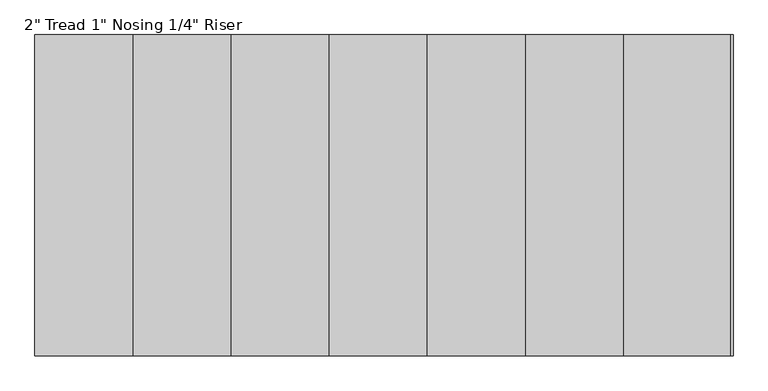
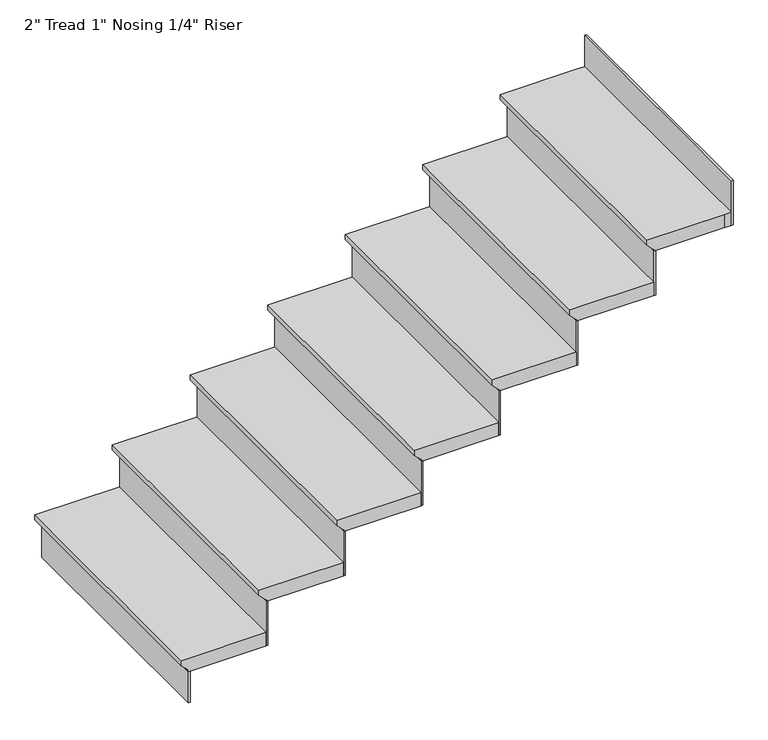
"""IFC4 building model written with IfcOpenShell, lengths in millimetres: stair flight geometry."""

from ifc_helpers import new_model, si_unit, origin, place, context, project, spatial, faceted_brep, source, transform, mapped, element, save


def stair_flight_2f37acb2(model_context):
    return source(origin(), model_context, "Body", "Brep", [
        faceted_brep([(-1404.564062, 2339.7857363, 6703.4833333), (-1404.564062, 2339.7857363, 6722.5333333), (-1404.564062, 3254.1857363, 6722.5333333), (-1404.564062, 3254.1857363, 6703.4833333), (-1379.164062, 2339.7857363, 6678.0833333), (-1379.164062, 3254.1857363, 6678.0833333), (-1099.764062, 2339.7857363, 6722.5333333), (-1099.764062, 3254.1857363, 6722.5333333), (-1379.164062, 3254.1857363, 6671.7333333), (-1099.764062, 3254.1857363, 6671.7333333), (-1099.764062, 2339.7857363, 6671.7333333), (-1379.164062, 2339.7857363, 6671.7333333)], [[[0, 1, 2, 3]], [[4, 0, 3, 5]], [[2, 1, 6, 7]], [[8, 9, 10, 11]], [[2, 7, 9, 8, 5, 3]], [[8, 11, 4, 5]], [[6, 1, 0, 4, 11, 10]], [[7, 6, 10, 9]]]),
        faceted_brep([(-1379.164062, 2339.7857363, 6671.7333333), (-1379.164062, 2339.7857363, 6553.2), (-1372.814062, 2339.7857363, 6553.2), (-1372.814062, 2339.7857363, 6671.7333333), (-1379.164062, 3254.1857363, 6671.7333333), (-1372.814062, 3254.1857363, 6671.7333333), (-1372.814062, 3254.1857363, 6553.2), (-1379.164062, 3254.1857363, 6553.2)], [[[0, 1, 2, 3]], [[4, 5, 6, 7]], [[1, 0, 4, 7]], [[2, 1, 7, 6]], [[3, 2, 6, 5]], [[0, 3, 5, 4]]]),
        faceted_brep([(-1099.764062, 2339.7857363, 6841.0666667), (-1099.764062, 2339.7857363, 6671.7333333), (-1093.414062, 2339.7857363, 6671.7333333), (-1093.414062, 2339.7857363, 6841.0666667), (-1099.764062, 3254.1857363, 6841.0666667), (-1093.414062, 3254.1857363, 6841.0666667), (-1093.414062, 3254.1857363, 6671.7333333), (-1099.764062, 3254.1857363, 6671.7333333)], [[[0, 1, 2, 3]], [[4, 5, 6, 7]], [[1, 0, 4, 7]], [[2, 1, 7, 6]], [[3, 2, 6, 5]], [[0, 3, 5, 4]]]),
        faceted_brep([(-1125.164062, 3254.1857363, 6891.8666667), (-1125.164062, 2339.7857363, 6891.8666667), (-820.364062, 2339.7857363, 6891.8666667), (-820.364062, 3254.1857363, 6891.8666667), (-1099.764062, 3254.1857363, 6841.0666667), (-820.364062, 3254.1857363, 6841.0666667), (-820.364062, 2339.7857363, 6841.0666667), (-1099.764062, 2339.7857363, 6841.0666667), (-1099.764062, 3254.1857363, 6847.4166667), (-1125.164062, 3254.1857363, 6872.8166667), (-1099.764062, 2339.7857363, 6847.4166667), (-1125.164062, 2339.7857363, 6872.8166667)], [[[0, 1, 2, 3]], [[4, 5, 6, 7]], [[0, 3, 5, 4, 8, 9]], [[4, 7, 10, 8]], [[2, 1, 11, 10, 7, 6]], [[3, 2, 6, 5]], [[11, 1, 0, 9]], [[10, 11, 9, 8]]]),
        faceted_brep([(-820.364062, 2339.7857363, 7010.4), (-820.364062, 2339.7857363, 6841.0666667), (-814.014062, 2339.7857363, 6841.0666667), (-814.014062, 2339.7857363, 7010.4), (-820.364062, 3254.1857363, 7010.4), (-814.014062, 3254.1857363, 7010.4), (-814.014062, 3254.1857363, 6841.0666667), (-820.364062, 3254.1857363, 6841.0666667)], [[[0, 1, 2, 3]], [[4, 5, 6, 7]], [[1, 0, 4, 7]], [[2, 1, 7, 6]], [[3, 2, 6, 5]], [[0, 3, 5, 4]]]),
        faceted_brep([(-845.764062, 3254.1857363, 7061.2), (-845.764062, 2339.7857363, 7061.2), (-540.964062, 2339.7857363, 7061.2), (-540.964062, 3254.1857363, 7061.2), (-820.364062, 3254.1857363, 7010.4), (-540.964062, 3254.1857363, 7010.4), (-540.964062, 2339.7857363, 7010.4), (-820.364062, 2339.7857363, 7010.4), (-820.364062, 3254.1857363, 7016.75), (-845.764062, 3254.1857363, 7042.15), (-820.364062, 2339.7857363, 7016.75), (-845.764062, 2339.7857363, 7042.15)], [[[0, 1, 2, 3]], [[4, 5, 6, 7]], [[0, 3, 5, 4, 8, 9]], [[4, 7, 10, 8]], [[2, 1, 11, 10, 7, 6]], [[3, 2, 6, 5]], [[11, 1, 0, 9]], [[10, 11, 9, 8]]]),
        faceted_brep([(-540.964062, 2339.7857363, 7179.7333333), (-540.964062, 2339.7857363, 7010.4), (-534.614062, 2339.7857363, 7010.4), (-534.614062, 2339.7857363, 7179.7333333), (-540.964062, 3254.1857363, 7179.7333333), (-534.614062, 3254.1857363, 7179.7333333), (-534.614062, 3254.1857363, 7010.4), (-540.964062, 3254.1857363, 7010.4)], [[[0, 1, 2, 3]], [[4, 5, 6, 7]], [[1, 0, 4, 7]], [[2, 1, 7, 6]], [[3, 2, 6, 5]], [[0, 3, 5, 4]]]),
        faceted_brep([(-566.364062, 3254.1857363, 7230.5333333), (-566.364062, 2339.7857363, 7230.5333333), (-261.564062, 2339.7857363, 7230.5333333), (-261.564062, 3254.1857363, 7230.5333333), (-540.964062, 3254.1857363, 7179.7333333), (-261.564062, 3254.1857363, 7179.7333333), (-261.564062, 2339.7857363, 7179.7333333), (-540.964062, 2339.7857363, 7179.7333333), (-540.964062, 3254.1857363, 7186.0833333), (-566.364062, 3254.1857363, 7211.4833333), (-540.964062, 2339.7857363, 7186.0833333), (-566.364062, 2339.7857363, 7211.4833333)], [[[0, 1, 2, 3]], [[4, 5, 6, 7]], [[0, 3, 5, 4, 8, 9]], [[4, 7, 10, 8]], [[2, 1, 11, 10, 7, 6]], [[3, 2, 6, 5]], [[11, 1, 0, 9]], [[10, 11, 9, 8]]]),
        faceted_brep([(-261.564062, 2339.7857363, 7349.0666667), (-261.564062, 2339.7857363, 7179.7333333), (-255.214062, 2339.7857363, 7179.7333333), (-255.214062, 2339.7857363, 7349.0666667), (-261.564062, 3254.1857363, 7349.0666667), (-255.214062, 3254.1857363, 7349.0666667), (-255.214062, 3254.1857363, 7179.7333333), (-261.564062, 3254.1857363, 7179.7333333)], [[[0, 1, 2, 3]], [[4, 5, 6, 7]], [[1, 0, 4, 7]], [[2, 1, 7, 6]], [[3, 2, 6, 5]], [[0, 3, 5, 4]]]),
        faceted_brep([(-286.964062, 3254.1857363, 7399.8666667), (-286.964062, 2339.7857363, 7399.8666667), (17.835938, 2339.7857363, 7399.8666667), (17.835938, 3254.1857363, 7399.8666667), (-261.564062, 3254.1857363, 7349.0666667), (17.835938, 3254.1857363, 7349.0666667), (17.835938, 2339.7857363, 7349.0666667), (-261.564062, 2339.7857363, 7349.0666667), (-261.564062, 3254.1857363, 7355.4166667), (-286.964062, 3254.1857363, 7380.8166667), (-261.564062, 2339.7857363, 7355.4166667), (-286.964062, 2339.7857363, 7380.8166667)], [[[0, 1, 2, 3]], [[4, 5, 6, 7]], [[0, 3, 5, 4, 8, 9]], [[4, 7, 10, 8]], [[2, 1, 11, 10, 7, 6]], [[3, 2, 6, 5]], [[11, 1, 0, 9]], [[10, 11, 9, 8]]]),
        faceted_brep([(17.835938, 2339.7857363, 7518.4), (17.835938, 2339.7857363, 7349.0666667), (24.185938, 2339.7857363, 7349.0666667), (24.185938, 2339.7857363, 7518.4), (17.835938, 3254.1857363, 7518.4), (24.185938, 3254.1857363, 7518.4), (24.185938, 3254.1857363, 7349.0666667), (17.835938, 3254.1857363, 7349.0666667)], [[[0, 1, 2, 3]], [[4, 5, 6, 7]], [[1, 0, 4, 7]], [[2, 1, 7, 6]], [[3, 2, 6, 5]], [[0, 3, 5, 4]]]),
        faceted_brep([(-7.564062, 3254.1857363, 7569.2), (-7.564062, 2339.7857363, 7569.2), (297.235938, 2339.7857363, 7569.2), (297.235938, 3254.1857363, 7569.2), (17.835938, 3254.1857363, 7518.4), (297.235938, 3254.1857363, 7518.4), (297.235938, 2339.7857363, 7518.4), (17.835938, 2339.7857363, 7518.4), (17.835938, 3254.1857363, 7524.75), (-7.564062, 3254.1857363, 7550.15), (17.835938, 2339.7857363, 7524.75), (-7.564062, 2339.7857363, 7550.15)], [[[0, 1, 2, 3]], [[4, 5, 6, 7]], [[0, 3, 5, 4, 8, 9]], [[4, 7, 10, 8]], [[2, 1, 11, 10, 7, 6]], [[3, 2, 6, 5]], [[11, 1, 0, 9]], [[10, 11, 9, 8]]]),
        faceted_brep([(576.635938, 2339.7857363, 7857.0666667), (576.635938, 2339.7857363, 7687.7333333), (582.985938, 2339.7857363, 7687.7333333), (582.985938, 2339.7857363, 7857.0666667), (576.635938, 3254.1857363, 7857.0666667), (582.985938, 3254.1857363, 7857.0666667), (582.985938, 3254.1857363, 7687.7333333), (576.635938, 3254.1857363, 7687.7333333)], [[[0, 1, 2, 3]], [[4, 5, 6, 7]], [[1, 0, 4, 7]], [[2, 1, 7, 6]], [[3, 2, 6, 5]], [[0, 3, 5, 4]]]),
        faceted_brep([(297.235938, 2339.7857363, 7687.7333333), (297.235938, 2339.7857363, 7518.4), (303.585938, 2339.7857363, 7518.4), (303.585938, 2339.7857363, 7687.7333333), (297.235938, 3254.1857363, 7687.7333333), (303.585938, 3254.1857363, 7687.7333333), (303.585938, 3254.1857363, 7518.4), (297.235938, 3254.1857363, 7518.4)], [[[0, 1, 2, 3]], [[4, 5, 6, 7]], [[1, 0, 4, 7]], [[2, 1, 7, 6]], [[3, 2, 6, 5]], [[0, 3, 5, 4]]]),
        faceted_brep([(576.635938, 3254.1857363, 7738.5333333), (551.235938, 3254.1857363, 7738.5333333), (271.835938, 3254.1857363, 7738.5333333), (271.835938, 2339.7857363, 7738.5333333), (551.235938, 2339.7857363, 7738.5333333), (576.635938, 2339.7857363, 7738.5333333), (551.235938, 3254.1857363, 7687.7333333), (576.635938, 3254.1857363, 7687.7333333), (576.635938, 2339.7857363, 7687.7333333), (551.235938, 2339.7857363, 7687.7333333), (297.235938, 2339.7857363, 7687.7333333), (297.235938, 3254.1857363, 7687.7333333), (297.235938, 3254.1857363, 7694.0833333), (271.835938, 3254.1857363, 7719.4833333), (297.235938, 2339.7857363, 7694.0833333), (271.835938, 2339.7857363, 7719.4833333)], [[[0, 1, 2, 3, 4, 5]], [[6, 7, 8, 9, 10, 11]], [[1, 0, 7, 6]], [[2, 1, 6, 11, 12, 13]], [[11, 10, 14, 12]], [[4, 3, 15, 14, 10, 9]], [[5, 4, 9, 8]], [[0, 5, 8, 7]], [[15, 3, 2, 13]], [[14, 15, 13, 12]]]),
    ])


if __name__ == "__main__":
    model = new_model("IFC4")
    model_context = context("Model", 3, world=origin())
    ifc_project = project(units=[si_unit("LENGTHUNIT", "METRE", prefix="MILLI")], contexts=[model_context])
    site = spatial("IfcSite", under=ifc_project)
    building = spatial("IfcBuilding", under=site)
    placement = place(None, origin())
    stair_flight_shape = stair_flight_2f37acb2(model_context)
    element("IfcStairFlight", 1, ObjectType="2\" Tread 1\" Nosing 1/4\" Riser", at=placement, inside=building, context=model_context, shape_type="MappedRepresentation", body=[
        mapped(stair_flight_shape, transform((0.0, 0.0, 0.0), x_axis=(1.0, 0.0, 0.0), y_axis=(0.0, 1.0, 0.0), z_axis=(0.0, 0.0, 1.0))),
    ])
    save(model, "model.ifc")

# Revit data of these elements
# Element 1 (IfcStairFlight, "2\" Tread 1\" Nosing 1/4\" Riser")
#   Materials on its faces: "BURGUNDY COLOUR"
# Materials
#   "BURGUNDY COLOUR": class "Generic", colour RGB 120 120 120, transparency 0, Cost = 0
